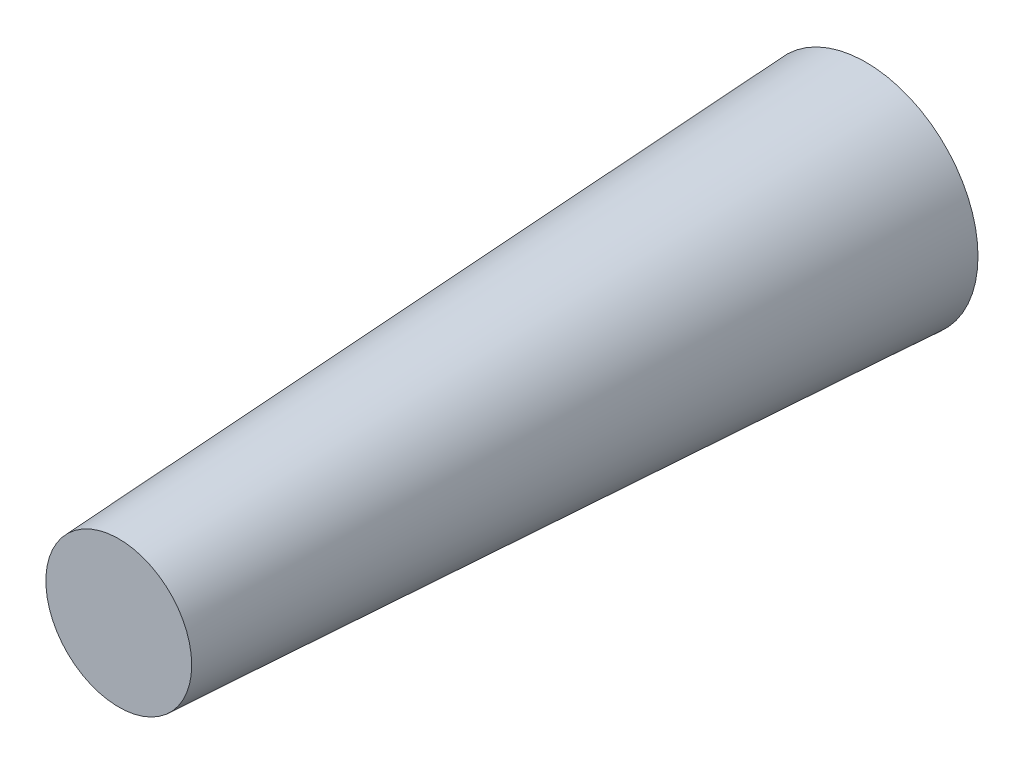
SolidWorks part; units mm, degrees
material "Plain Carbon Steel"
ref_plane "Front Plane" through (0, 0, 0) normal (0, 0, 1) x (1, 0, 0)
ref_plane "Top Plane" through (0, 0, 0) normal (0, 1, 0) x (1, 0, 0)
ref_plane "Right Plane" through (0, 0, 0) normal (1, 0, 0) x (0, 0, -1)
sketch "Pin Profile Ø6" plane through (0, 0, 0) normal (0, 0, 1) x (1, 0, 0)
  circle A0 centre (0, 0) radius 3
  dimension "D1" = 6
extrude "Taper Pin Body 20mm 3° Draft" add sketch "Pin Profile Ø6" along normal blind 20 draft 3
